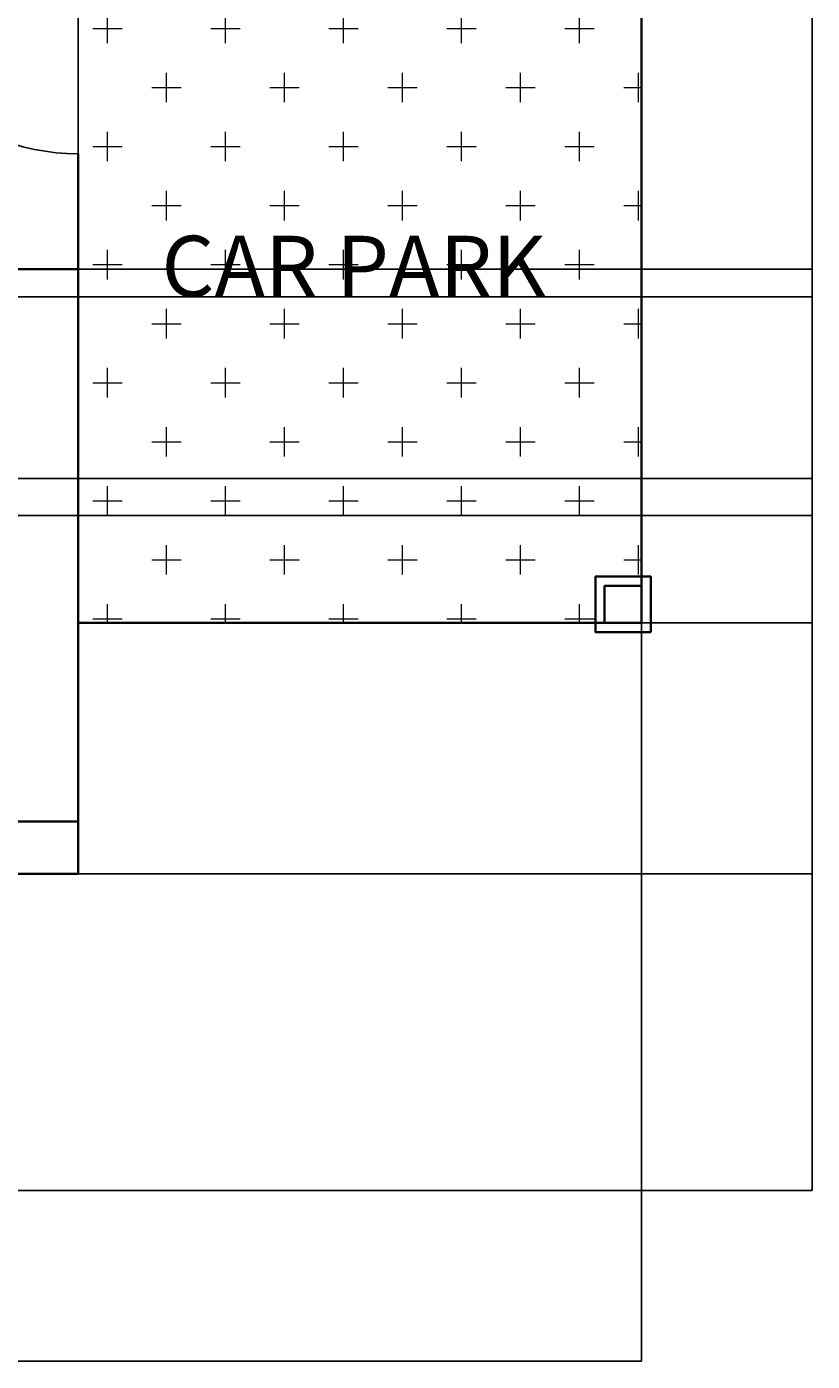
# Model space of a CAD drawing. Units: millimetres. Extents: x 19292 to 100733, y 12374 to 26974.
# Tile 16 of 24: x 33498 to 36880, y 12809 to 18550. Entities that reach past the tile are written whole.
import ezdxf

# ---------------------------------------------------------------- set-up
doc = ezdxf.new("R2010")
doc.units = ezdxf.units.MM
for name, color, linetype, lineweight in [('A-ANNO-DIMS', 2, 'Continuous', 18), ('A-AREA-IDEN', 3, 'Continuous', 25), ('A-DOOR', 4, 'Continuous', 25), ('A-FLOR-PATT', 252, 'Continuous', 13), ('A-WALL', 7, 'Continuous', 35)]:
    doc.layers.add(name, color=color, linetype=linetype, lineweight=lineweight)
doc.styles.get("Standard").update_dxf_attribs({"font": 'arial.ttf'})
doc.dimstyles.get("Standard").update_dxf_attribs({"dimtxt": 0.18, "dimasz": 0.18, "dimexe": 0.18, "dimexo": 0.0625, "dimgap": 0.09, "dimtad": 0, "dimtih": 1, "dimtoh": 1, "dimdec": 4, "dimzin": 0, "dimdsep": 46, "dimtxsty": 'Standard', "dimcen": 0.09, "dimadec": 0, "dimazin": 0, "dimtfac": 1, "dimtdec": 4, "dimtofl": 0, "dimtmove": 0, "dimatfit": 3, "dimfxl": 1, "dimtolj": 1, "dimtzin": 0, "dimarcsym": 0})

# ---------------------------------------------------------------- blocks, each defined once
blk = doc.blocks.new('DOOR-900')
for p, q in [((927.7, 80), (0, 80)), ((927.7, 0), (927.7, 80)), ((927.7, 0), (927.7, 80)), ((927.7, 0), (0, 0))]:
    blk.add_line(p, q)
blk.add_arc((927.7, 0), 927.7, 90, 180)
blk = doc.blocks.new('*D70')
at = {"layer": 'A-ANNO-DIMS', "color": 0, "lineweight": -2, "transparency": 16777216}
for p, q in [((23573.9, 17387.7), (36879.3, 17387.7)), ((36879.2, 17387.6), (36879.2, 16917.9)), ((36879.2, 16447.9), (36879.2, 16917.6)), ((23573.9, 16447.7), (36879.3, 16447.7))]:
    blk.add_line(p, q, dxfattribs=at)
at = {"layer": 'A-ANNO-DIMS', "color": 0, "transparency": 16777216}
for points in [[(36879.1, 17387.6), (36879.2, 17387.6), (36879.2, 17387.7)], [(36879.1, 16447.9), (36879.2, 16447.9), (36879.2, 16447.7)]]:
    blk.add_solid(points, dxfattribs=at)
at = {"layer": 'Defpoints', "color": 0, "transparency": 16777216}
for p in [(23573.8, 17387.7), (36879.2, 17387.7), (23573.8, 16447.7)]:
    blk.add_point(p, dxfattribs=at)
at = {"layer": 'A-ANNO-DIMS', "color": 0, "transparency": 16777216, "insert": (36879.2, 16917.7), "char_height": 0.18, "attachment_point": 5}
blk.add_mtext('\\A1;940', dxfattribs=at)
blk = doc.blocks.new('*D72')
at = {"layer": 'A-ANNO-DIMS', "color": 0, "lineweight": -2, "transparency": 16777216}
for p, q in [((33719.9, 14906.4), (36879.3, 14906.4)), ((36879.2, 14906.2), (36879.2, 14225.4)), ((36879.2, 13544.2), (36879.2, 14225)), ((31394.9, 13544), (36879.3, 13544))]:
    blk.add_line(p, q, dxfattribs=at)
at = {"layer": 'A-ANNO-DIMS', "color": 0, "transparency": 16777216}
for points in [[(36879.1, 14906.2), (36879.2, 14906.2), (36879.2, 14906.4)], [(36879.1, 13544.2), (36879.2, 13544.2), (36879.2, 13544)]]:
    blk.add_solid(points, dxfattribs=at)
at = {"layer": 'Defpoints', "color": 0, "transparency": 16777216}
for p in [(33719.8, 14906.4), (36879.2, 14906.4), (31394.8, 13544)]:
    blk.add_point(p, dxfattribs=at)
at = {"layer": 'A-ANNO-DIMS', "color": 0, "transparency": 16777216, "insert": (36879.2, 14225.2), "char_height": 0.18, "attachment_point": 5}
blk.add_mtext('\\A1;1362.4', dxfattribs=at)
blk = doc.blocks.new('*D73')
at = {"layer": 'A-ANNO-DIMS', "color": 0, "lineweight": -2, "transparency": 16777216}
for p, q in [((36144.2, 15985.7), (36879.3, 15985.7)), ((36879.2, 15985.5), (36879.2, 15446.2)), ((36879.2, 14906.6), (36879.2, 15445.9)), ((33719.9, 14906.4), (36879.3, 14906.4))]:
    blk.add_line(p, q, dxfattribs=at)
at = {"layer": 'A-ANNO-DIMS', "color": 0, "transparency": 16777216}
for points in [[(36879.1, 15985.5), (36879.2, 15985.5), (36879.2, 15985.7)], [(36879.1, 14906.6), (36879.2, 14906.6), (36879.2, 14906.4)]]:
    blk.add_solid(points, dxfattribs=at)
at = {"layer": 'Defpoints', "color": 0, "transparency": 16777216}
for p in [(36144.2, 15985.7), (36879.2, 15985.7), (33719.8, 14906.4)]:
    blk.add_point(p, dxfattribs=at)
at = {"layer": 'A-ANNO-DIMS', "color": 0, "transparency": 16777216, "insert": (36879.2, 15446.1), "char_height": 0.18, "attachment_point": 5}
blk.add_mtext('\\A1;1079.3', dxfattribs=at)
blk = doc.blocks.new('*D74')
at = {"layer": 'A-ANNO-DIMS', "color": 0, "lineweight": -2, "transparency": 16777216}
for p, q in [((36144.2, 19010.7), (36879.3, 19010.7)), ((36879.2, 19010.5), (36879.2, 17498.4)), ((36879.2, 15985.9), (36879.2, 17498)), ((36144.2, 15985.7), (36879.3, 15985.7))]:
    blk.add_line(p, q, dxfattribs=at)
at = {"layer": 'A-ANNO-DIMS', "color": 0, "transparency": 16777216}
for points in [[(36879.1, 19010.5), (36879.2, 19010.5), (36879.2, 19010.7)], [(36879.1, 15985.9), (36879.2, 15985.9), (36879.2, 15985.7)]]:
    blk.add_solid(points, dxfattribs=at)
at = {"layer": 'Defpoints', "color": 0, "transparency": 16777216}
for p in [(36144.2, 19010.7), (36879.2, 19010.7), (36144.2, 15985.7)]:
    blk.add_point(p, dxfattribs=at)
at = {"layer": 'A-ANNO-DIMS', "color": 0, "transparency": 16777216, "insert": (36879.2, 17498.2), "char_height": 0.18, "attachment_point": 5}
blk.add_mtext('\\A1;3025', dxfattribs=at)
blk = doc.blocks.new('*D79')
at = {"layer": 'A-ANNO-DIMS', "color": 0, "lineweight": -2, "transparency": 16777216}
for p, q in [((22694.1, 22860.7), (22694.1, 12808.8)), ((36144.2, 15985.7), (36144.2, 12808.8)), ((22694.3, 12809), (29418.7, 12809)), ((36144, 12809), (29419.6, 12809))]:
    blk.add_line(p, q, dxfattribs=at)
at = {"layer": 'A-ANNO-DIMS', "color": 0, "transparency": 16777216}
for points in [[(22694.3, 12809), (22694.3, 12809), (22694.1, 12809)], [(36144, 12809), (36144, 12809), (36144.2, 12809)]]:
    blk.add_solid(points, dxfattribs=at)
at = {"layer": 'Defpoints', "color": 0, "transparency": 16777216}
for p in [(22694.1, 22860.7), (36144.2, 15985.7), (36144.2, 12809)]:
    blk.add_point(p, dxfattribs=at)
at = {"layer": 'A-ANNO-DIMS', "color": 0, "transparency": 16777216, "insert": (29419.2, 12809), "char_height": 0.18, "attachment_point": 5}
blk.add_mtext('\\A1;13450', dxfattribs=at)
blk = doc.blocks.new('*D84')
at = {"layer": 'A-ANNO-DIMS', "color": 0, "lineweight": -2, "transparency": 16777216}
for p, q in [((33719.2, 15985.8), (33719.2, 23555.9)), ((33719.3, 23555.7), (34931.3, 23555.7)), ((36144, 23555.7), (34932, 23555.7)), ((36144.2, 15985.8), (36144.2, 23555.9))]:
    blk.add_line(p, q, dxfattribs=at)
at = {"layer": 'A-ANNO-DIMS', "color": 0, "transparency": 16777216}
for points in [[(33719.3, 23555.8), (33719.3, 23555.7), (33719.2, 23555.7)], [(36144, 23555.8), (36144, 23555.7), (36144.2, 23555.7)]]:
    blk.add_solid(points, dxfattribs=at)
at = {"layer": 'Defpoints', "color": 0, "transparency": 16777216}
for p in [(36144.2, 23555.7), (33719.2, 15985.7), (36144.2, 15985.7)]:
    blk.add_point(p, dxfattribs=at)
at = {"layer": 'A-ANNO-DIMS', "color": 0, "transparency": 16777216, "insert": (34931.7, 23555.7), "char_height": 0.18, "attachment_point": 5}
blk.add_mtext('\\A1;2425', dxfattribs=at)
blk = doc.blocks.new('*D89')
at = {"layer": 'A-ANNO-DIMS', "color": 0, "lineweight": -2, "transparency": 16777216}
for p, q in [((31394.9, 17506.4), (36879.3, 17506.4)), ((36879.2, 17506.2), (36879.2, 17056.6)), ((36879.2, 16606.6), (36879.2, 17056.2)), ((31394.9, 16606.4), (36879.3, 16606.4))]:
    blk.add_line(p, q, dxfattribs=at)
at = {"layer": 'A-ANNO-DIMS', "color": 0, "transparency": 16777216}
for points in [[(36879.1, 17506.2), (36879.2, 17506.2), (36879.2, 17506.4)], [(36879.1, 16606.6), (36879.2, 16606.6), (36879.2, 16606.4)]]:
    blk.add_solid(points, dxfattribs=at)
at = {"layer": 'Defpoints', "color": 0, "transparency": 16777216}
for p in [(31394.8, 17506.4), (31394.8, 16606.4), (36879.2, 16606.4)]:
    blk.add_point(p, dxfattribs=at)
at = {"layer": 'A-ANNO-DIMS', "color": 0, "transparency": 16777216, "insert": (36879.2, 17056.4), "char_height": 0.18, "attachment_point": 5}
blk.add_mtext('\\A1;900', dxfattribs=at)

msp = doc.modelspace()

# ---------------------------------------------------------------- hatches: boundary and pattern name
at = {"layer": 'A-FLOR-PATT'}
h = msp.add_hatch(dxfattribs=at)
h.set_pattern_fill('CROSS', color=256, scale=40)
h.paths.add_polyline_path([(36144.169, 19010.725), (33719.169, 19010.725), (33719.169, 18850.725), (33719.169, 18003.026), (33719.169, 15985.725), (36144.169, 15985.725)])
h.paths.add_polyline_path([(36144.132, 22460.725), (34419.132, 22460.725), (34419.132, 22208.026, -0.34415073), (35121.831, 21308.026), (34419.132, 21308.026), (34419.132, 21260.725), (36144.132, 21260.725)])
h.paths.add_polyline_path([(34419.132, 22208.026), (34419.132, 21388.026), (35118.375, 21388.026, 0.32018294)], flags=17)
h.paths.add_polyline_path([(31169.132, 22460.725), (28369.132, 22460.725), (28369.132, 21460.725), (31169.132, 21460.725)])
h.paths.add_polyline_path([(34010.406, 17316.149), (36018.156, 17316.149), (36018.156, 17722.778), (34010.406, 17722.778)], flags=24)
h.paths.add_polyline_path([(34456.896, 21920.301), (35605.434, 21920.301), (35605.434, 22313.518), (34456.896, 22313.518)], flags=25)
h.paths.add_polyline_path([(29263.068, 21823.707), (30421.489, 21823.707), (30421.489, 22034.008), (29263.068, 22034.008)], flags=24)

# ---------------------------------------------------------------- linework, layer by layer
at = {"layer": 'A-WALL'}
for points in [[(33719.169, 18850.725), (33719.169, 19010.725), (36144.169, 19010.725), (36144.169, 15985.725), (33719.169, 15985.725), (33719.169, 18003.026)], [(31969.132, 17506.403), (31619.799, 17506.403), (31619.799, 15131.403), (33719.799, 15131.403), (33719.799, 17506.403), (33369.132, 17506.403)], [(33719.66, 15985.725), (33719.835, 14906.403), (31051.542, 14906.403)]]:
    msp.add_lwpolyline(points, dxfattribs=at)
for points in [[(36184.169, 15945.725), (35945.717, 15945.725), (35945.717, 16184.177), (36184.169, 16184.177)], [(36144.169, 15985.725), (35985.717, 15985.725), (35985.717, 16144.177), (36144.169, 16144.177)]]:
    msp.add_lwpolyline(points, close=True, dxfattribs=at)

# ---------------------------------------------------------------- block references
at = {"layer": 'A-DOOR', "extrusion": (0, 0, -1), "zscale": -1, "rotation": 180}
msp.add_blockref('DOOR-900', (-32791.471, 18930.725), dxfattribs=at)

# ---------------------------------------------------------------- texts
at = {"layer": 'A-AREA-IDEN'}
msp.add_text('CAR PARK', height=262.1447, dxfattribs=at).set_placement((34078.178, 17388.391))

# ---------------------------------------------------------------- dimensions: what is measured, and where the dimension line sits
at = {"layer": 'A-ANNO-DIMS'}
for base, p1, picture, middle in [((36144.169, 23555.725), (33719.169, 15985.725), '*D84', (34931.669, 23555.725)), ((36144.169, 12808.993), (22694.132, 22860.725), '*D79', (29419.151, 12808.993))]:
    dim = msp.add_linear_dim(base=base, p1=p1, p2=(36144.169, 15985.725), dimstyle='Standard', override={"dimdec": 0, "dimlfac": 1, "dimrnd": 0, "dimzin": 0, "dimdsep": 46, "dimlunit": 2}, dxfattribs=at)
    dim.commit()
    dim.dimension.update_dxf_attribs({"geometry": picture, "text_midpoint": middle})
for base, p1, p2, override, picture, middle in [((36879.169, 19010.725), (36144.169, 15985.725), (36144.169, 19010.725), {"dimdec": 0, "dimlfac": 1, "dimrnd": 0, "dimzin": 0, "dimdsep": 46, "dimlunit": 2}, '*D74', (36879.169, 17498.225)), ((36879.169, 16606.403), (31394.799, 17506.403), (31394.799, 16606.403), {"dimdec": 0, "dimlfac": 1, "dimrnd": 0, "dimzin": 0, "dimdsep": 46, "dimlunit": 2}, '*D89', (36879.169, 17056.403)), ((36879.169, 17387.748), (23573.815, 16447.748), (23573.815, 17387.748), {"dimdec": 0, "dimlfac": 1, "dimrnd": 0, "dimzin": 0, "dimdsep": 46, "dimlunit": 2}, '*D70', (36879.169, 16917.748)), ((36879.169, 15985.725), (33719.835, 14906.403), (36144.169, 15985.725), {"dimdec": 1, "dimlfac": 1, "dimrnd": 0, "dimzin": 0, "dimdsep": 46, "dimlunit": 2}, '*D73', (36879.169, 15446.064)), ((36879.169, 14906.403), (31394.799, 13543.993), (33719.835, 14906.403), {"dimdec": 1, "dimlfac": 1, "dimrnd": 0, "dimzin": 0, "dimdsep": 46, "dimlunit": 2}, '*D72', (36879.169, 14225.198))]:
    dim = msp.add_linear_dim(base=base, p1=p1, p2=p2, angle=90, dimstyle='Standard', override=override, dxfattribs=at)
    dim.commit()
    dim.dimension.update_dxf_attribs({"geometry": picture, "text_midpoint": middle})

doc.saveas('drawing.dxf')
